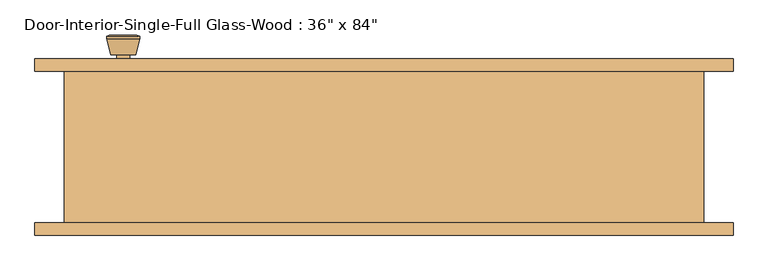
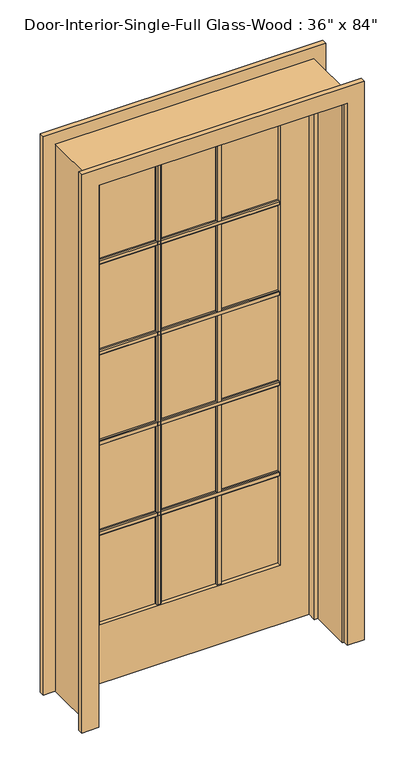
"""IFC4 building model written with IfcOpenShell, lengths in millimetres: door geometry."""

from ifc_helpers import new_model, si_unit, point, frame, frame_2d, origin, place, context, project, spatial, polyline, circle_curve, trimmed, segment, composite_curve, outline, extrude, faceted_brep, source, transform, mapped, element, save
from ifc_brep_helpers import plane_surface, cylinder_surface, revolved_surface, advanced_brep


def door_c89e1556(model_context):
    return source(origin(), model_context, "Body", "SolidModel", [
        extrude(outline(polyline([(97.155, 1667.51), (103.505, 1667.51), (106.68, 1664.335), (106.68, 1651.635), (103.505, 1648.46), (97.155, 1648.46), (97.155, 1667.51)])), frame((-336.55, 0.0, 0.0), z_axis=(1.0, 0.0, 0.0), x_axis=(0.0, 1.0, 0.0)), (0.0, 0.0, 1.0), 673.1),
        extrude(outline(polyline([(97.155, 1310.9575), (103.505, 1310.9575), (106.68, 1307.7825), (106.68, 1295.0825), (103.505, 1291.9075), (97.155, 1291.9075), (97.155, 1310.9575)])), frame((-336.55, 0.0, 0.0), z_axis=(1.0, 0.0, 0.0), x_axis=(0.0, 1.0, 0.0)), (0.0, 0.0, 1.0), 673.1),
        extrude(outline(polyline([(97.155, 954.405), (103.505, 954.405), (106.68, 951.23), (106.68, 938.53), (103.505, 935.355), (97.155, 935.355), (97.155, 954.405)])), frame((-336.55, 0.0, 0.0), z_axis=(1.0, 0.0, 0.0), x_axis=(0.0, 1.0, 0.0)), (0.0, 0.0, 1.0), 673.1),
        extrude(outline(polyline([(97.155, 597.8525), (103.505, 597.8525), (106.68, 594.6775), (106.68, 581.9775), (103.505, 578.8025), (97.155, 578.8025), (97.155, 597.8525)])), frame((-336.55, 0.0, 0.0), z_axis=(1.0, 0.0, 0.0), x_axis=(0.0, 1.0, 0.0)), (0.0, 0.0, 1.0), 673.1),
        extrude(outline(polyline([(102.6583333, 97.155), (102.6583333, 103.505), (105.8333333, 106.68), (118.5333333, 106.68), (121.7083333, 103.505), (121.7083333, 97.155), (102.6583333, 97.155)])), frame((0.0, 0.0, 231.775), z_axis=(0.0, 0.0, 1.0), x_axis=(1.0, 0.0, 0.0)), (0.0, 0.0, 1.0), 1782.7625),
        extrude(outline(polyline([(-121.7083333, 97.155), (-121.7083333, 103.505), (-118.5333333, 106.68), (-105.8333333, 106.68), (-102.6583333, 103.505), (-102.6583333, 97.155), (-121.7083333, 97.155)])), frame((0.0, 0.0, 231.775), z_axis=(0.0, 0.0, 1.0), x_axis=(1.0, 0.0, 0.0)), (0.0, 0.0, 1.0), 1782.7625),
        extrude(outline(polyline([(90.17, 1667.51), (90.17, 1648.46), (83.82, 1648.46), (80.645, 1651.635), (80.645, 1664.335), (83.82, 1667.51), (90.17, 1667.51)])), frame((-336.55, 0.0, 0.0), z_axis=(1.0, 0.0, 0.0), x_axis=(0.0, 1.0, 0.0)), (0.0, 0.0, 1.0), 673.1),
        extrude(outline(polyline([(90.17, 1310.9575), (90.17, 1291.9075), (83.82, 1291.9075), (80.645, 1295.0825), (80.645, 1307.7825), (83.82, 1310.9575), (90.17, 1310.9575)])), frame((-336.55, 0.0, 0.0), z_axis=(1.0, 0.0, 0.0), x_axis=(0.0, 1.0, 0.0)), (0.0, 0.0, 1.0), 673.1),
        extrude(outline(polyline([(90.17, 954.405), (90.17, 935.355), (83.82, 935.355), (80.645, 938.53), (80.645, 951.23), (83.82, 954.405), (90.17, 954.405)])), frame((-336.55, 0.0, 0.0), z_axis=(1.0, 0.0, 0.0), x_axis=(0.0, 1.0, 0.0)), (0.0, 0.0, 1.0), 673.1),
        extrude(outline(polyline([(90.17, 597.8525), (90.17, 578.8025), (83.82, 578.8025), (80.645, 581.9775), (80.645, 594.6775), (83.82, 597.8525), (90.17, 597.8525)])), frame((-336.55, 0.0, 0.0), z_axis=(1.0, 0.0, 0.0), x_axis=(0.0, 1.0, 0.0)), (0.0, 0.0, 1.0), 673.1),
        extrude(outline(polyline([(102.6583333, 90.17), (121.7083333, 90.17), (121.7083333, 83.82), (118.5333333, 80.645), (105.8333333, 80.645), (102.6583333, 83.82), (102.6583333, 90.17)])), frame((0.0, 0.0, 231.775), z_axis=(0.0, 0.0, 1.0), x_axis=(1.0, 0.0, 0.0)), (0.0, 0.0, 1.0), 1782.7625),
        extrude(outline(polyline([(-121.7083333, 90.17), (-102.6583333, 90.17), (-102.6583333, 83.82), (-105.8333333, 80.645), (-118.5333333, 80.645), (-121.7083333, 83.82), (-121.7083333, 90.17)])), frame((0.0, 0.0, 231.775), z_axis=(0.0, 0.0, 1.0), x_axis=(1.0, 0.0, 0.0)), (0.0, 0.0, 1.0), 1782.7625),
        advanced_brep(
        [(-393.7, 70.2, 914.4), (-383.7, 70.2, 914.4), (-403.7, 70.2, 914.4), (-373.2241324, 21.2, 914.4), (-393.7, 21.2, 914.4), (-414.1758676, 21.2, 914.4), (-368.7, 23.0278681, 914.4), (-418.7, 23.0278681, 914.4), (-368.7, 26.4915463, 914.4), (-418.7, 26.4915463, 914.4), (-375.063764, 51.2, 914.4), (-412.336236, 51.2, 914.4), (-383.7, 51.2, 914.4), (-403.7, 51.2, 914.4)],
        [
            (0, 1),
            (1, 2, circle_curve(frame((-393.7, 70.2, 914.4), z_axis=(0.0, 1.0, 0.0), x_axis=(-1.0, 0.0, 0.0)), 10.0)),
            (2, 0),
            (2, 1, circle_curve(frame((-393.7, 70.2, 914.4), z_axis=(0.0, 1.0, 0.0), x_axis=(-1.0, 0.0, 0.0)), 10.0)),
            (3, 4),
            (4, 5),
            (5, 3, circle_curve(frame((-393.7, 21.2, 914.4), z_axis=(0.0, -1.0, 0.0), x_axis=(-1.0, 0.0, 0.0)), 20.4758676)),
            (3, 5, circle_curve(frame((-393.7, 21.2, 914.4), z_axis=(0.0, -1.0, 0.0), x_axis=(-1.0, 0.0, 0.0)), 20.4758676)),
            (6, 3),
            (5, 7),
            (7, 6, circle_curve(frame((-393.7, 23.0278681, 914.4), z_axis=(0.0, -1.0, 0.0), x_axis=(-1.0, 0.0, 0.0)), 25.0)),
            (6, 7, circle_curve(frame((-393.7, 23.0278681, 914.4), z_axis=(0.0, -1.0, 0.0), x_axis=(-1.0, 0.0, 0.0)), 25.0)),
            (8, 6),
            (7, 9),
            (9, 8, circle_curve(frame((-393.7, 26.4915463, 914.4), z_axis=(0.0, -1.0, 0.0), x_axis=(-1.0, 0.0, 0.0)), 25.0)),
            (8, 9, circle_curve(frame((-393.7, 26.4915463, 914.4), z_axis=(0.0, -1.0, 0.0), x_axis=(-1.0, 0.0, 0.0)), 25.0)),
            (10, 8),
            (9, 11),
            (11, 10, circle_curve(frame((-393.7, 51.2, 914.4), z_axis=(0.0, -1.0, 0.0), x_axis=(-1.0, 0.0, 0.0)), 18.636236)),
            (10, 11, circle_curve(frame((-393.7, 51.2, 914.4), z_axis=(0.0, -1.0, 0.0), x_axis=(-1.0, 0.0, 0.0)), 18.636236)),
            (12, 10),
            (11, 13),
            (13, 12, circle_curve(frame((-393.7, 51.2, 914.4), z_axis=(0.0, -1.0, 0.0), x_axis=(-1.0, 0.0, 0.0)), 10.0)),
            (12, 13, circle_curve(frame((-393.7, 51.2, 914.4), z_axis=(0.0, -1.0, 0.0), x_axis=(-1.0, 0.0, 0.0)), 10.0)),
            (1, 12),
            (13, 2),
        ],
        [
            plane_surface(frame((-393.7, 70.2, 914.4), z_axis=(0.0, 1.0, 0.0), x_axis=(-1.0, 0.0, 0.0))),
            plane_surface(frame((-393.7, 21.2, 914.4), z_axis=(0.0, -1.0, 0.0), x_axis=(-1.0, 0.0, 0.0))),
            revolved_surface(polyline([(-414.1758676, 21.2, 914.4), (-418.7, 23.0278681, 914.4)]), (-393.7, 70.2, 914.4), (0.0, 1.0, 0.0)),
            cylinder_surface(frame((-393.7, 70.2, 914.4), z_axis=(0.0, 1.0, 0.0), x_axis=(-1.0, 0.0, 0.0)), 25.0),
            revolved_surface(polyline([(-418.7, 26.4915463, 914.4), (-412.336236, 51.2, 914.4)]), (-393.7, 70.2, 914.4), (0.0, 1.0, 0.0)),
            plane_surface(frame((-393.7, 51.2, 914.4), z_axis=(0.0, 1.0, 0.0), x_axis=(-1.0, 0.0, 0.0))),
            cylinder_surface(frame((-393.7, 70.2, 914.4), z_axis=(0.0, 1.0, 0.0), x_axis=(-1.0, 0.0, 0.0)), 10.0),
        ],
        [
            (0, [[1, 2, 3]]),
            (0, [[-3, 4, -1]]),
            (1, [[5, 6, 7]]),
            (1, [[-6, -5, 8]]),
            (2, [[9, -7, 10, 11]]),
            (2, [[-10, -8, -9, 12]]),
            (3, [[13, -11, 14, 15]]),
            (3, [[-14, -12, -13, 16]]),
            (4, [[17, -15, 18, 19]]),
            (4, [[-18, -16, -17, 20]]),
            (5, [[21, -19, 22, 23]]),
            (5, [[-22, -20, -21, 24]]),
            (6, [[25, -23, 26, -2]]),
            (6, [[-26, -24, -25, -4]]),
        ],
    ),
        extrude(outline(composite_curve([segment(trimmed(circle_curve(frame_2d((914.4, -393.7)), 30.0), [point((914.4, -423.7))], [point((914.4, -363.7))], False, "CARTESIAN"), True, "CONTINUOUS"), segment(trimmed(circle_curve(frame_2d((914.4, -393.7)), 30.0), [point((914.4, -363.7))], [point((914.4, -423.7))], False, "CARTESIAN"), True, "CONTINUOUS")], self_intersect=False)), frame((0.0, 70.2, 0.0), z_axis=(0.0, 1.0, 0.0), x_axis=(0.0, 0.0, 1.0)), (0.0, 0.0, 1.0), 6.0),
        advanced_brep(
        [(-393.7, 117.125, 914.4), (-403.7, 117.125, 914.4), (-383.7, 117.125, 914.4), (-373.2241324, 166.125, 914.4), (-414.1758676, 166.125, 914.4), (-393.7, 166.125, 914.4), (-368.7, 164.2971319, 914.4), (-418.7, 164.2971319, 914.4), (-368.7, 160.8334537, 914.4), (-418.7, 160.8334537, 914.4), (-375.063764, 136.125, 914.4), (-412.336236, 136.125, 914.4), (-383.7, 136.125, 914.4), (-403.7, 136.125, 914.4)],
        [
            (0, 1),
            (1, 2, circle_curve(frame((-393.7, 117.125, 914.4), z_axis=(0.0, -1.0, 0.0), x_axis=(-1.0, 0.0, 0.0)), 10.0)),
            (2, 0),
            (2, 1, circle_curve(frame((-393.7, 117.125, 914.4), z_axis=(0.0, -1.0, 0.0), x_axis=(-1.0, 0.0, 0.0)), 10.0)),
            (3, 4, circle_curve(frame((-393.7, 166.125, 914.4), z_axis=(0.0, 1.0, 0.0), x_axis=(-1.0, 0.0, 0.0)), 20.4758676)),
            (4, 5),
            (5, 3),
            (4, 3, circle_curve(frame((-393.7, 166.125, 914.4), z_axis=(0.0, 1.0, 0.0), x_axis=(-1.0, 0.0, 0.0)), 20.4758676)),
            (6, 7, circle_curve(frame((-393.7, 164.2971319, 914.4), z_axis=(0.0, 1.0, 0.0), x_axis=(-1.0, 0.0, 0.0)), 25.0)),
            (7, 4),
            (3, 6),
            (7, 6, circle_curve(frame((-393.7, 164.2971319, 914.4), z_axis=(0.0, 1.0, 0.0), x_axis=(-1.0, 0.0, 0.0)), 25.0)),
            (8, 9, circle_curve(frame((-393.7, 160.8334537, 914.4), z_axis=(0.0, 1.0, 0.0), x_axis=(-1.0, 0.0, 0.0)), 25.0)),
            (9, 7),
            (6, 8),
            (9, 8, circle_curve(frame((-393.7, 160.8334537, 914.4), z_axis=(0.0, 1.0, 0.0), x_axis=(-1.0, 0.0, 0.0)), 25.0)),
            (10, 11, circle_curve(frame((-393.7, 136.125, 914.4), z_axis=(0.0, 1.0, 0.0), x_axis=(-1.0, 0.0, 0.0)), 18.636236)),
            (11, 9),
            (8, 10),
            (11, 10, circle_curve(frame((-393.7, 136.125, 914.4), z_axis=(0.0, 1.0, 0.0), x_axis=(-1.0, 0.0, 0.0)), 18.636236)),
            (12, 13, circle_curve(frame((-393.7, 136.125, 914.4), z_axis=(0.0, 1.0, 0.0), x_axis=(-1.0, 0.0, 0.0)), 10.0)),
            (13, 11),
            (10, 12),
            (13, 12, circle_curve(frame((-393.7, 136.125, 914.4), z_axis=(0.0, 1.0, 0.0), x_axis=(-1.0, 0.0, 0.0)), 10.0)),
            (1, 13),
            (12, 2),
        ],
        [
            plane_surface(frame((-393.7, 117.125, 914.4), z_axis=(0.0, -1.0, 0.0), x_axis=(-1.0, 0.0, 0.0))),
            plane_surface(frame((-393.7, 166.125, 914.4), z_axis=(0.0, 1.0, 0.0), x_axis=(-1.0, 0.0, 0.0))),
            revolved_surface(polyline([(-414.1758676, 166.125, 914.4), (-418.7, 164.2971319, 914.4)]), (-393.7, 117.125, 914.4), (0.0, -1.0, 0.0)),
            cylinder_surface(frame((-393.7, 117.125, 914.4), z_axis=(0.0, -1.0, 0.0), x_axis=(-1.0, 0.0, 0.0)), 25.0),
            revolved_surface(polyline([(-418.7, 160.8334537, 914.4), (-412.336236, 136.125, 914.4)]), (-393.7, 117.125, 914.4), (0.0, -1.0, 0.0)),
            plane_surface(frame((-393.7, 136.125, 914.4), z_axis=(0.0, -1.0, 0.0), x_axis=(-1.0, 0.0, 0.0))),
            cylinder_surface(frame((-393.7, 117.125, 914.4), z_axis=(0.0, -1.0, 0.0), x_axis=(-1.0, 0.0, 0.0)), 10.0),
        ],
        [
            (0, [[1, 2, 3]]),
            (0, [[-3, 4, -1]]),
            (1, [[5, 6, 7]]),
            (1, [[8, -7, -6]]),
            (2, [[9, 10, -5, 11]]),
            (2, [[12, -11, -8, -10]]),
            (3, [[13, 14, -9, 15]]),
            (3, [[16, -15, -12, -14]]),
            (4, [[17, 18, -13, 19]]),
            (4, [[20, -19, -16, -18]]),
            (5, [[21, 22, -17, 23]]),
            (5, [[24, -23, -20, -22]]),
            (6, [[-2, 25, -21, 26]]),
            (6, [[-4, -26, -24, -25]]),
        ],
    ),
        extrude(outline(composite_curve([segment(trimmed(circle_curve(frame_2d((914.4, -393.7)), 30.0), [point((914.4, -423.7))], [point((914.4, -363.7))], False, "CARTESIAN"), True, "CONTINUOUS"), segment(trimmed(circle_curve(frame_2d((914.4, -393.7)), 30.0), [point((914.4, -363.7))], [point((914.4, -423.7))], False, "CARTESIAN"), True, "CONTINUOUS")], self_intersect=False)), frame((0.0, 111.125, 0.0), z_axis=(0.0, 1.0, 0.0), x_axis=(0.0, 0.0, 1.0)), (0.0, 0.0, 1.0), 6.0),
        faceted_brep([(482.6, 111.125, 0.0), (482.6, -117.475, 0.0), (457.2, -117.475, 0.0), (457.2, 41.275, 0.0), (444.5, 41.275, 0.0), (444.5, 76.2, 0.0), (457.2, 76.2, 0.0), (457.2, 111.125, 0.0), (482.6, 111.125, 2159.0), (482.6, -117.475, 2159.0), (-482.6, -117.475, 2159.0), (-482.6, -117.475, 0.0), (-457.2, -117.475, 0.0), (-457.2, -117.475, 2133.6), (457.2, -117.475, 2133.6), (457.2, 41.275, 2133.6), (-457.2, 41.275, 2133.6), (-457.2, 41.275, 0.0), (-444.5, 41.275, 0.0), (-444.5, 41.275, 2120.9), (444.5, 41.275, 2120.9), (444.5, 76.2, 2120.9), (-444.5, 76.2, 2120.9), (-444.5, 76.2, 0.0), (-457.2, 76.2, 0.0), (-457.2, 76.2, 2133.6), (457.2, 76.2, 2133.6), (457.2, 111.125, 2133.6), (-457.2, 111.125, 2133.6), (-457.2, 111.125, 0.0), (-482.6, 111.125, 0.0), (-482.6, 111.125, 2159.0)], [[[0, 1, 2, 3, 4, 5, 6, 7]], [[1, 0, 8, 9]], [[2, 1, 9, 10, 11, 12, 13, 14]], [[3, 2, 14, 15]], [[4, 3, 15, 16, 17, 18, 19, 20]], [[5, 4, 20, 21]], [[6, 5, 21, 22, 23, 24, 25, 26]], [[7, 6, 26, 27]], [[0, 7, 27, 28, 29, 30, 31, 8]], [[9, 8, 31, 10]], [[15, 14, 13, 16]], [[21, 20, 19, 22]], [[27, 26, 25, 28]], [[30, 29, 24, 23, 18, 17, 12, 11]], [[10, 31, 30, 11]], [[16, 13, 12, 17]], [[22, 19, 18, 23]], [[28, 25, 24, 29]]]),
        extrude(outline(polyline([(2133.6, -457.2), (0.0, -457.2), (0.0, 457.2), (2133.6, 457.2), (2133.6, -457.2)]), holes=[polyline([(2014.5375, -336.55), (2014.5375, 336.55), (231.775, 336.55), (231.775, -336.55), (2014.5375, -336.55)])]), frame((0.0, 76.2, 0.0), z_axis=(0.0, 1.0, 0.0), x_axis=(0.0, 0.0, 1.0)), (0.0, 0.0, 1.0), 34.925),
        extrude(outline(polyline([(336.55, 90.17), (-336.55, 90.17), (-336.55, 97.155), (336.55, 97.155), (336.55, 90.17)])), frame((0.0, 0.0, 231.775), z_axis=(0.0, 0.0, 1.0), x_axis=(1.0, 0.0, 0.0)), (0.0, 0.0, 1.0), 1782.7625),
        extrude(outline(polyline([(0.0, 463.55), (0.0, 527.05), (2203.45, 527.05), (2203.45, -527.05), (0.0, -527.05), (0.0, -463.55), (2139.95, -463.55), (2139.95, 463.55), (0.0, 463.55)])), frame((0.0, 111.125, 0.0), z_axis=(0.0, 1.0, 0.0), x_axis=(0.0, 0.0, 1.0)), (0.0, 0.0, 1.0), 19.05),
        extrude(outline(polyline([(0.0, 463.55), (0.0, 527.05), (2203.45, 527.05), (2203.45, -527.05), (0.0, -527.05), (0.0, -463.55), (2139.95, -463.55), (2139.95, 463.55), (0.0, 463.55)])), frame((0.0, -136.525, 0.0), z_axis=(0.0, 1.0, 0.0), x_axis=(0.0, 0.0, 1.0)), (0.0, 0.0, 1.0), 19.05),
    ])


if __name__ == "__main__":
    model = new_model("IFC4")
    model_context = context("Model", 3, world=origin())
    ifc_project = project(units=[si_unit("LENGTHUNIT", "METRE", prefix="MILLI")], contexts=[model_context])
    site = spatial("IfcSite", under=ifc_project)
    building = spatial("IfcBuilding", under=site)
    placement = place(None, origin())
    door_shape = door_c89e1556(model_context)
    element("IfcDoor", 1, ObjectType="Door-Interior-Single-Full Glass-Wood : 36\" x 84\"", at=placement, inside=building, context=model_context, shape_type="MappedRepresentation", body=[
        mapped(door_shape, transform((0.0, 0.0, 0.0), x_axis=(1.0, 0.0, 0.0), y_axis=(0.0, 1.0, 0.0), z_axis=(0.0, 0.0, 1.0))),
    ])
    save(model, "model.ifc")

# Revit data of these elements
# Type "Door-Interior-Single-Full Glass-Wood : 36\" x 84\""
#   Type Mark = "8"
#   Assembly Code = "C1020300"
#   Analytic Construction = "Wood frame with single clear glass"
#   Top Rail = 0' - 4 11/16"
#   Thickness = 0' - 1 3/8"
#   Thermal Resistance (R) = 1.0102 (h·ft²·°F)/BTU
#   Swing Angle [instance default] = 90.00°
#   Stiles = 0' - 4 3/4"
#   Rough Width = 3' - 2"
#   Rough Height = 7' - 1"
#   Height = 7' - 0"
#   Width = 3' - 0"
#   Heat Transfer Coefficient (U) = 0.9900 BTU/(h·ft²·°F)
#   Bottom Rail = 0' - 9 1/8"
#   Show Grill [instance default] = yes
#   Trim Material = Cherry
#   Panel Material = Cherry
#   Frame Material = Cherry
#   Door Handle Material = Aluminum
#   Visual Light Transmittance = 0
#   Solar Heat Gain Coefficient = 0
#   Wall Closure = (empty or 0)
#   Function = (empty or 0)
# Element 1 (IfcDoor, "Door-Interior-Single-Full Glass-Wood : 36\" x 84\"")
#   Materials on its faces: "Cherry", "Aluminum", "Glass"
# Materials
#   "Cherry": class "Wood", colour RGB 226 177 128, transparency 0, Description = "Prunus Serotina", Cost = 0
#   "Aluminum": class "Metal", colour RGB 247 247 247, transparency 0, Description = "Aluminum 6061", Cost = 0
#   "Glass": class "Glass", colour RGB 0 128 192, transparency 0.75, Description = "Soda Lime Glass", Cost = 0
